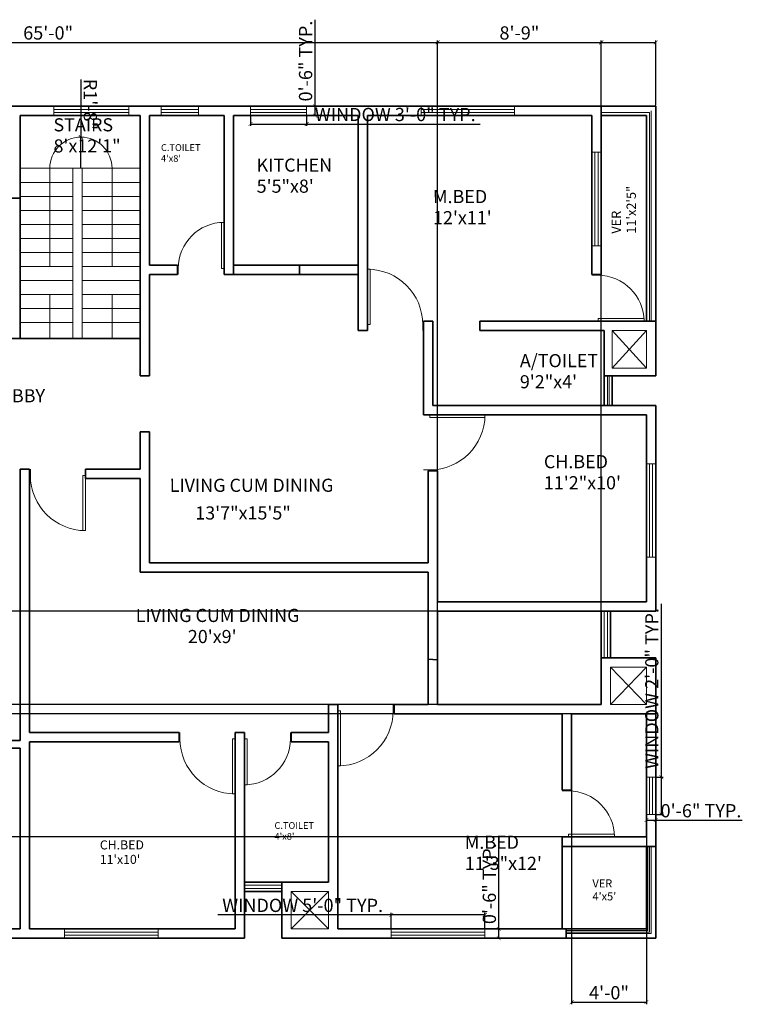
# Model space of a CAD drawing. Units: inches. Extents: x 3799 to 20199, y 1682 to 8087.
# Tile 3 of 30: x 6616 to 7080, y 1729 to 2361. Entities that reach past the tile are written whole.
import ezdxf

# ---------------------------------------------------------------- set-up
doc = ezdxf.new("R2010")
doc.units = ezdxf.units.IN
for name, color, linetype, lineweight in [('A-ANNO-DIMS', 2, 'Continuous', 18), ('A-AREA-IDEN', 7, 'Continuous', 18), ('A-DOOR', 3, 'Continuous', 18), ('A-FLOR-RAIL', 217, 'Continuous', 18), ('A-FLOR-SHFT', 8, 'Continuous', 18), ('A-FLOR-STRS', 41, 'Continuous', 18), ('A-GLAZ', 152, 'Continuous', 18), ('A-WALL', 7, 'Continuous', 35)]:
    doc.layers.add(name, color=color, linetype=linetype, lineweight=lineweight)
doc.styles.get("Standard").update_dxf_attribs({"font": 'arial.ttf'})
doc.dimstyles.new('ISO-25', dxfattribs={"dimtxt": 8.5, "dimasz": 2.5, "dimexe": 1.25, "dimexo": 0.625, "dimtad": 1, "dimdec": 0, "dimlunit": 3, "dimtxsty": 'Standard', "dimblk": 'ARCHTICK', "dimcen": 2.5, "dimadec": 0, "dimazin": 0, "dimtfac": 1, "dimtdec": 0, "dimtmove": 0, "dimatfit": 3, "dimfxl": 1, "dimarcsym": 0})

# ---------------------------------------------------------------- blocks, each defined once
blk = doc.blocks.new('*U16')
for p, q in [((0, 0), (0, -100)), ((900, 0), (900, -100))]:
    blk.add_line(p, q)
blk.add_lwpolyline([(0, 0), (0, 900), (43.75, 900), (43.75, 0)], close=True)
blk.add_arc((0, 0), 900, 0, 90)
blk = doc.blocks.new('*U17')
for p, q in [((-750, 0), (-750, -100)), ((0, 0), (0, -100))]:
    blk.add_line(p, q)
blk.add_lwpolyline([(0, 0), (0, 750), (-43.75, 750), (-43.75, 0)], close=True)
blk.add_arc((0, 0), 750, 90, 180)
blk = doc.blocks.new('*U11')
for p, q in [((-900, 0), (-900, 100)), ((0, 0), (0, 100))]:
    blk.add_line(p, q)
blk.add_lwpolyline([(0, 0), (0, -900), (-43.75, -900), (-43.75, 0)], close=True)
blk.add_arc((0, 0), 900, 180, 270)
blk = doc.blocks.new('*U13')
for p, q in [((0, 0), (0, 100)), ((750, 0), (750, 100))]:
    blk.add_line(p, q)
blk.add_lwpolyline([(0, 0), (0, -750), (43.75, -750), (43.75, 0)], close=True)
blk.add_arc((0, 0), 750, 270, 0)
blk = doc.blocks.new('*U14')
for p, q in [((0, 0), (0, 100)), ((900, 0), (900, 100))]:
    blk.add_line(p, q)
blk.add_lwpolyline([(0, 0), (0, -900), (43.75, -900), (43.75, 0)], close=True)
blk.add_arc((0, 0), 900, 270, 0)
blk = doc.blocks.new('*U15')
for p, q in [((0, 0), (0, 100)), ((750, 0), (750, 100))]:
    blk.add_line(p, q)
blk.add_lwpolyline([(0, 0), (0, -750), (43.75, -750), (43.75, 0)], close=True)
blk.add_arc((0, 0), 750, 270, 0)
blk = doc.blocks.new('*U18')
for p, q in [((-900, 0), (-900, 100)), ((0, 0), (0, 100))]:
    blk.add_line(p, q)
blk.add_lwpolyline([(0, 0), (0, -900), (-43.75, -900), (-43.75, 0)], close=True)
blk.add_arc((0, 0), 900, 180, 270)
blk = doc.blocks.new('*U19')
for p, q in [((0, 0), (0, 100)), ((750, 0), (750, 100))]:
    blk.add_line(p, q)
blk.add_lwpolyline([(0, 0), (0, -750), (43.75, -750), (43.75, 0)], close=True)
blk.add_arc((0, 0), 750, 270, 0)
blk = doc.blocks.new('WIN-60IN-6IN-FRAME')
for p, q in [((6, 60), (0, 60)), ((2, 60), (2, 0)), ((4, 60), (4, 0)), ((6, 0), (0, 0))]:
    blk.add_line(p, q)
blk = doc.blocks.new('WIN-24IN-6IN-FRAME')
for p, q in [((6, 24), (0, 24)), ((2, 24), (2, 0)), ((4, 24), (4, 0)), ((6, 0), (0, 0))]:
    blk.add_line(p, q)
blk = doc.blocks.new('WIN-48IN-6IN-FRAME')
for p, q in [((0, 0), (0, 6)), ((48, 4), (0, 4)), ((48, 2), (0, 2)), ((48, 0), (48, 6))]:
    blk.add_line(p, q)
blk = doc.blocks.new('WIN-36IN-6IN-FRAME')
for p, q in [((0, 0), (0, 6)), ((36, 4), (0, 4)), ((36, 2), (0, 2)), ((36, 0), (36, 6))]:
    blk.add_line(p, q)
blk = doc.blocks.new('SHAFT-24X24IN')
for p, q in [((0, 24), (0, 0)), ((24, 24), (0, 24)), ((0, 24), (24, 0)), ((0, 0), (24, 24)), ((24, 24), (24, 0)), ((0, 0), (24, 0))]:
    blk.add_line(p, q)
blk = doc.blocks.new('_ArchTick')
at = {"color": 0, "linetype": 'ByBlock', "const_width": 0.15}
blk.add_lwpolyline([(-0.5, -0.5), (0.5, 0.5)], dxfattribs=at)
blk = doc.blocks.new('*D268')
at = {"layer": 'A-ANNO-DIMS', "color": 0, "lineweight": -2, "transparency": 16777216}
for p, q in [((6854.93, 1786.05), (6743.62, 1786.05)), ((6854.93, 1777.67), (6854.93, 1787.3)), ((6914.93, 1786.05), (6854.93, 1786.05)), ((6914.93, 1777.67), (6914.93, 1787.3))]:
    blk.add_line(p, q, dxfattribs=at)
at = {"layer": 'Defpoints', "color": 0, "transparency": 16777216}
for p in [(6854.93, 1786.05), (6854.93, 1777.05), (6914.93, 1777.05)]:
    blk.add_point(p, dxfattribs=at)
at = {"layer": 'A-ANNO-DIMS', "color": 0, "lineweight": -2, "transparency": 16777216, "xscale": 2.5, "yscale": 2.5, "zscale": 2.5, "rotation": 180}
blk.add_blockref('_ArchTick', (6854.93, 1786.05), dxfattribs=at)
at = {"layer": 'A-ANNO-DIMS', "color": 0, "lineweight": -2, "transparency": 16777216, "xscale": 2.5, "yscale": 2.5, "zscale": 2.5}
blk.add_blockref('_ArchTick', (6914.93, 1786.05), dxfattribs=at)
at = {"layer": 'A-ANNO-DIMS', "color": 0, "transparency": 16777216, "insert": (6798.02, 1791.07), "char_height": 8.5, "attachment_point": 5}
blk.add_mtext('WINDOW 5\'-0" TYP.', dxfattribs=at)
blk = doc.blocks.new('*D269')
at = {"layer": 'A-ANNO-DIMS', "color": 0, "lineweight": -2, "transparency": 16777216}
for p, q in [((6923.93, 1777.05), (6923.93, 1832.61)), ((6915.55, 1777.05), (6925.18, 1777.05)), ((6923.93, 1771.05), (6923.93, 1777.05)), ((6915.55, 1771.05), (6925.18, 1771.05))]:
    blk.add_line(p, q, dxfattribs=at)
at = {"layer": 'Defpoints', "color": 0, "transparency": 16777216}
for p in [(6914.93, 1777.05), (6923.93, 1777.05), (6914.93, 1771.05)]:
    blk.add_point(p, dxfattribs=at)
at = {"layer": 'A-ANNO-DIMS', "color": 0, "lineweight": -2, "transparency": 16777216, "xscale": 2.5, "yscale": 2.5, "zscale": 2.5}
for p, rotation in [((6923.93, 1777.05), 90), ((6923.93, 1771.05), 270)]:
    blk.add_blockref('_ArchTick', p, dxfattribs=dict(at, rotation=rotation))
at = {"layer": 'A-ANNO-DIMS', "color": 0, "transparency": 16777216, "insert": (6918.96, 1806.08), "char_height": 8.5, "attachment_point": 5, "rotation": 90}
blk.add_mtext('0\'-6" TYP.', dxfattribs=at)
blk = doc.blocks.new('*D310')
at = {"layer": 'A-ANNO-DIMS', "color": 0, "lineweight": -2, "transparency": 16777216}
for p, q in [((7028.27, 1874.46), (7028.27, 1985.77)), ((7025.3, 1874.46), (7029.52, 1874.46)), ((7028.27, 1850.46), (7028.27, 1874.46)), ((7025.3, 1850.46), (7029.52, 1850.46))]:
    blk.add_line(p, q, dxfattribs=at)
at = {"layer": 'Defpoints', "color": 0, "transparency": 16777216}
for p in [(7024.67, 1874.46), (7028.27, 1874.46), (7024.67, 1850.46)]:
    blk.add_point(p, dxfattribs=at)
at = {"layer": 'A-ANNO-DIMS', "color": 0, "lineweight": -2, "transparency": 16777216, "xscale": 2.5, "yscale": 2.5, "zscale": 2.5}
for p, rotation in [((7028.27, 1874.46), 90), ((7028.27, 1850.46), 270)]:
    blk.add_blockref('_ArchTick', p, dxfattribs=dict(at, rotation=rotation))
at = {"layer": 'A-ANNO-DIMS', "color": 0, "transparency": 16777216, "insert": (7023.25, 1931.36), "char_height": 8.5, "attachment_point": 5, "rotation": 90}
blk.add_mtext('WINDOW 2\'-0" TYP.', dxfattribs=at)
blk = doc.blocks.new('*D311')
at = {"layer": 'A-ANNO-DIMS', "color": 0, "lineweight": -2, "transparency": 16777216}
for p, q in [((7018.67, 1849.83), (7018.67, 1845.61)), ((7018.67, 1846.86), (7024.67, 1846.86)), ((7024.67, 1849.83), (7024.67, 1845.61)), ((7024.67, 1846.86), (7080.24, 1846.86))]:
    blk.add_line(p, q, dxfattribs=at)
at = {"layer": 'Defpoints', "color": 0, "transparency": 16777216}
for p in [(7018.67, 1850.46), (7024.67, 1850.46), (7024.67, 1846.86)]:
    blk.add_point(p, dxfattribs=at)
at = {"layer": 'A-ANNO-DIMS', "color": 0, "lineweight": -2, "transparency": 16777216, "xscale": 2.5, "yscale": 2.5, "zscale": 2.5, "rotation": 180}
blk.add_blockref('_ArchTick', (7018.67, 1846.86), dxfattribs=at)
at = {"layer": 'A-ANNO-DIMS', "color": 0, "lineweight": -2, "transparency": 16777216, "xscale": 2.5, "yscale": 2.5, "zscale": 2.5}
blk.add_blockref('_ArchTick', (7024.67, 1846.86), dxfattribs=at)
at = {"layer": 'A-ANNO-DIMS', "color": 0, "transparency": 16777216, "insert": (7053.71, 1851.82), "char_height": 8.5, "attachment_point": 5}
blk.add_mtext('0\'-6" TYP.', dxfattribs=at)
blk = doc.blocks.new('*D336')
at = {"layer": 'A-ANNO-DIMS', "color": 0, "lineweight": -2, "transparency": 16777216}
for p, q in [((6764.57, 2298.42), (6764.57, 2292.4)), ((6800.57, 2298.42), (6800.57, 2292.4)), ((6764.57, 2293.65), (6800.57, 2293.65)), ((6800.57, 2293.65), (6911.88, 2293.65))]:
    blk.add_line(p, q, dxfattribs=at)
at = {"layer": 'Defpoints', "color": 0, "transparency": 16777216}
for p in [(6764.57, 2299.05), (6800.57, 2299.05), (6800.57, 2293.65)]:
    blk.add_point(p, dxfattribs=at)
at = {"layer": 'A-ANNO-DIMS', "color": 0, "lineweight": -2, "transparency": 16777216, "xscale": 2.5, "yscale": 2.5, "zscale": 2.5, "rotation": 180}
blk.add_blockref('_ArchTick', (6764.57, 2293.65), dxfattribs=at)
at = {"layer": 'A-ANNO-DIMS', "color": 0, "lineweight": -2, "transparency": 16777216, "xscale": 2.5, "yscale": 2.5, "zscale": 2.5}
blk.add_blockref('_ArchTick', (6800.57, 2293.65), dxfattribs=at)
at = {"layer": 'A-ANNO-DIMS', "color": 0, "transparency": 16777216, "insert": (6857.47, 2298.67), "char_height": 8.5, "attachment_point": 5}
blk.add_mtext('WINDOW 3\'-0" TYP.', dxfattribs=at)
blk = doc.blocks.new('*D337')
at = {"layer": 'A-ANNO-DIMS', "color": 0, "lineweight": -2, "transparency": 16777216}
for p, q in [((6805.97, 2305.05), (6805.97, 2360.61)), ((6801.19, 2305.05), (6807.22, 2305.05)), ((6805.97, 2299.05), (6805.97, 2305.05)), ((6801.19, 2299.05), (6807.22, 2299.05))]:
    blk.add_line(p, q, dxfattribs=at)
at = {"layer": 'Defpoints', "color": 0, "transparency": 16777216}
for p in [(6800.57, 2305.05), (6805.97, 2305.05), (6800.57, 2299.05)]:
    blk.add_point(p, dxfattribs=at)
at = {"layer": 'A-ANNO-DIMS', "color": 0, "lineweight": -2, "transparency": 16777216, "xscale": 2.5, "yscale": 2.5, "zscale": 2.5}
for p, rotation in [((6805.97, 2305.05), 90), ((6805.97, 2299.05), 270)]:
    blk.add_blockref('_ArchTick', p, dxfattribs=dict(at, rotation=rotation))
at = {"layer": 'A-ANNO-DIMS', "color": 0, "transparency": 16777216, "insert": (6801, 2334.08), "char_height": 8.5, "attachment_point": 5, "rotation": 90}
blk.add_mtext('0\'-6" TYP.', dxfattribs=at)
blk = doc.blocks.new('*D356')
at = {"layer": 'A-ANNO-DIMS', "color": 0, "lineweight": -2, "transparency": 16777216}
for p, q in [((6244.67, 2305.67), (6244.67, 2347.3)), ((6244.67, 2346.05), (7024.67, 2346.05)), ((7024.67, 2305.67), (7024.67, 2347.3))]:
    blk.add_line(p, q, dxfattribs=at)
at = {"layer": 'Defpoints', "color": 0, "transparency": 16777216}
for p in [(7024.67, 2346.05), (6244.67, 2305.05), (7024.67, 2305.05)]:
    blk.add_point(p, dxfattribs=at)
at = {"layer": 'A-ANNO-DIMS', "color": 0, "lineweight": -2, "transparency": 16777216, "xscale": 2.5, "yscale": 2.5, "zscale": 2.5, "rotation": 180}
blk.add_blockref('_ArchTick', (6244.67, 2346.05), dxfattribs=at)
at = {"layer": 'A-ANNO-DIMS', "color": 0, "lineweight": -2, "transparency": 16777216, "xscale": 2.5, "yscale": 2.5, "zscale": 2.5}
blk.add_blockref('_ArchTick', (7024.67, 2346.05), dxfattribs=at)
at = {"layer": 'A-ANNO-DIMS', "color": 0, "transparency": 16777216, "insert": (6634.67, 2351.01), "char_height": 8.5, "attachment_point": 5}
blk.add_mtext('65\'-0"', dxfattribs=at)
blk = doc.blocks.new('*D367')
at = {"layer": 'A-ANNO-DIMS', "color": 0, "lineweight": -2, "transparency": 16777216}
for p, q in [((6884.67, 1921.67), (6884.67, 2347.3)), ((6884.67, 2346.05), (6989.67, 2346.05)), ((6989.67, 1921.67), (6989.67, 2347.3))]:
    blk.add_line(p, q, dxfattribs=at)
at = {"layer": 'Defpoints', "color": 0, "transparency": 16777216}
for p in [(6989.67, 2346.05), (6884.67, 1921.05), (6989.67, 1921.05)]:
    blk.add_point(p, dxfattribs=at)
at = {"layer": 'A-ANNO-DIMS', "color": 0, "lineweight": -2, "transparency": 16777216, "xscale": 2.5, "yscale": 2.5, "zscale": 2.5, "rotation": 180}
blk.add_blockref('_ArchTick', (6884.67, 2346.05), dxfattribs=at)
at = {"layer": 'A-ANNO-DIMS', "color": 0, "lineweight": -2, "transparency": 16777216, "xscale": 2.5, "yscale": 2.5, "zscale": 2.5}
blk.add_blockref('_ArchTick', (6989.67, 2346.05), dxfattribs=at)
at = {"layer": 'A-ANNO-DIMS', "color": 0, "transparency": 16777216, "insert": (6937.17, 2351.01), "char_height": 8.5, "attachment_point": 5}
blk.add_mtext('8\'-9"', dxfattribs=at)
blk = doc.blocks.new('*D368')
at = {"layer": 'A-ANNO-DIMS', "color": 0, "lineweight": -2, "transparency": 16777216}
for p, q in [((6989.05, 1981.05), (6202.42, 1981.05)), ((6203.67, 1921.05), (6203.67, 1981.05)), ((6989.05, 1921.05), (6202.42, 1921.05))]:
    blk.add_line(p, q, dxfattribs=at)
at = {"layer": 'Defpoints', "color": 0, "transparency": 16777216}
for p in [(6203.67, 1981.05), (6989.67, 1981.05), (6989.67, 1921.05)]:
    blk.add_point(p, dxfattribs=at)
at = {"layer": 'A-ANNO-DIMS', "color": 0, "lineweight": -2, "transparency": 16777216, "xscale": 2.5, "yscale": 2.5, "zscale": 2.5}
for p, rotation in [((6203.67, 1981.05), 90), ((6203.67, 1921.05), 270)]:
    blk.add_blockref('_ArchTick', p, dxfattribs=dict(at, rotation=rotation))
at = {"layer": 'A-ANNO-DIMS', "color": 0, "transparency": 16777216, "insert": (6198.71, 1951.05), "char_height": 8.5, "attachment_point": 5, "rotation": 90}
blk.add_mtext('5\'-0"', dxfattribs=at)
blk = doc.blocks.new('*D369')
at = {"layer": 'A-ANNO-DIMS', "color": 0, "lineweight": -2, "transparency": 16777216}
for p, q in [((6970.67, 1914.42), (6970.67, 1728.8)), ((7018.67, 1914.42), (7018.67, 1728.8)), ((6970.67, 1730.05), (7018.67, 1730.05))]:
    blk.add_line(p, q, dxfattribs=at)
at = {"layer": 'Defpoints', "color": 0, "transparency": 16777216}
for p in [(6970.67, 1915.05), (7018.67, 1915.05), (7018.67, 1730.05)]:
    blk.add_point(p, dxfattribs=at)
at = {"layer": 'A-ANNO-DIMS', "color": 0, "lineweight": -2, "transparency": 16777216, "xscale": 2.5, "yscale": 2.5, "zscale": 2.5, "rotation": 180}
blk.add_blockref('_ArchTick', (6970.67, 1730.05), dxfattribs=at)
at = {"layer": 'A-ANNO-DIMS', "color": 0, "lineweight": -2, "transparency": 16777216, "xscale": 2.5, "yscale": 2.5, "zscale": 2.5}
blk.add_blockref('_ArchTick', (7018.67, 1730.05), dxfattribs=at)
at = {"layer": 'A-ANNO-DIMS', "color": 0, "transparency": 16777216, "insert": (6994.67, 1735.01), "char_height": 8.5, "attachment_point": 5}
blk.add_mtext('4\'-0"', dxfattribs=at)
blk = doc.blocks.new('*D370')
at = {"layer": 'A-ANNO-DIMS', "color": 0, "lineweight": -2, "transparency": 16777216}
for p, q in [((7018.05, 1915.05), (6202.42, 1915.05)), ((6203.67, 1836.05), (6203.67, 1915.05)), ((7018.05, 1836.05), (6202.42, 1836.05))]:
    blk.add_line(p, q, dxfattribs=at)
at = {"layer": 'Defpoints', "color": 0, "transparency": 16777216}
for p in [(6203.67, 1915.05), (7018.67, 1915.05), (7018.67, 1836.05)]:
    blk.add_point(p, dxfattribs=at)
at = {"layer": 'A-ANNO-DIMS', "color": 0, "lineweight": -2, "transparency": 16777216, "xscale": 2.5, "yscale": 2.5, "zscale": 2.5}
for p, rotation in [((6203.67, 1915.05), 90), ((6203.67, 1836.05), 270)]:
    blk.add_blockref('_ArchTick', p, dxfattribs=dict(at, rotation=rotation))
at = {"layer": 'A-ANNO-DIMS', "color": 0, "transparency": 16777216, "insert": (6198.71, 1875.55), "char_height": 8.5, "attachment_point": 5, "rotation": 90}
blk.add_mtext('6\'-7"', dxfattribs=at)
blk = doc.blocks.new('*D385')
at = {"layer": 'A-ANNO-DIMS', "color": 0, "lineweight": -2, "transparency": 16777216}
for p in [(6655.67, 2322.2), (6655.68, 2265.22)]:
    blk.add_line(p, (6655.68, 2285.22), dxfattribs=at)
at = {"layer": 'Defpoints', "color": 0, "transparency": 16777216}
for p in [(6655.68, 2285.22), (6655.68, 2265.22)]:
    blk.add_point(p, dxfattribs=at)
at = {"layer": 'A-ANNO-DIMS', "color": 0, "lineweight": -2, "transparency": 16777216, "xscale": 2.5, "yscale": 2.5, "zscale": 2.5, "rotation": 270.0003322570112}
blk.add_blockref('_ArchTick', (6655.68, 2285.22), dxfattribs=at)
at = {"layer": 'A-ANNO-DIMS', "color": 0, "transparency": 16777216, "insert": (6660.64, 2306.21), "char_height": 8.5, "attachment_point": 5, "rotation": 270.00033}
blk.add_mtext('R1\'-8"', dxfattribs=at)

msp = doc.modelspace()

# ---------------------------------------------------------------- linework, layer by layer
at = {"layer": 'A-FLOR-RAIL'}
for p, q in [((7020.67, 2301.05), (6989.67, 2301.05)), ((7020.67, 2167.05), (7020.67, 2301.05)), ((7021.67, 2167.05), (7021.67, 2302.05)), ((7019.67, 1776.05), (7019.67, 1830.05)), ((7020.67, 1775.05), (7020.67, 1830.05)), ((7021.67, 1774.05), (7021.67, 1830.05)), ((6967.17, 1776.05), (7019.67, 1776.05)), ((6967.17, 1775.05), (7020.67, 1775.05)), ((6967.17, 1775.05), (7018.67, 1775.05)), ((6967.17, 1774.05), (7021.67, 1774.05))]:
    msp.add_line(p, q, dxfattribs=at)
at = {"layer": 'A-FLOR-SHFT'}
for p, q in [((7018.67, 2161.05), (6996.67, 2161.05)), ((6996.67, 2161.05), (6996.67, 2137.05)), ((6996.67, 2161.05), (7018.67, 2137.05)), ((7018.67, 2161.05), (6996.67, 2137.05)), ((7018.67, 2161.05), (7018.67, 2137.05)), ((7018.67, 2137.05), (6996.67, 2137.05)), ((7018.67, 1945.05), (6995.67, 1945.05)), ((6995.67, 1945.05), (6995.67, 1921.05)), ((6995.67, 1945.05), (7018.67, 1921.05)), ((6995.67, 1921.05), (7018.67, 1945.05)), ((7018.67, 1921.05), (7018.67, 1945.05)), ((7018.67, 1921.05), (6995.67, 1921.05))]:
    msp.add_line(p, q, dxfattribs=at)
at = {"layer": 'A-FLOR-STRS'}
for p, q in [((6616.67, 2265.22), (6693.67, 2265.22)), ((6635.67, 2265.22), (6635.67, 2202.22)), ((6650.58, 2265.22), (6650.58, 2156.05)), ((6656.58, 2265.22), (6656.58, 2156.05)), ((6675.68, 2265.22), (6675.68, 2202.22)), ((6616.67, 2256.22), (6650.58, 2256.22)), ((6656.58, 2256.22), (6693.67, 2256.22)), ((6616.67, 2247.22), (6650.58, 2247.22)), ((6656.58, 2247.22), (6693.67, 2247.22)), ((6616.67, 2238.22), (6650.58, 2238.22)), ((6656.58, 2238.22), (6693.67, 2238.22)), ((6616.67, 2229.22), (6650.58, 2229.22)), ((6656.58, 2229.22), (6693.67, 2229.22)), ((6616.67, 2220.22), (6650.58, 2220.22)), ((6656.58, 2220.22), (6693.67, 2220.22)), ((6616.67, 2211.22), (6650.58, 2211.22)), ((6656.58, 2211.22), (6693.67, 2211.22)), ((6616.67, 2202.22), (6650.58, 2202.22)), ((6656.58, 2202.22), (6693.67, 2202.22)), ((6616.67, 2193.22), (6650.58, 2193.22)), ((6656.58, 2193.22), (6693.67, 2193.22)), ((6616.67, 2184.22), (6650.58, 2184.22)), ((6635.67, 2184.22), (6635.67, 2156.05)), ((6656.58, 2184.22), (6693.67, 2184.22)), ((6675.68, 2184.22), (6675.68, 2156.05)), ((6616.67, 2175.22), (6650.58, 2175.22)), ((6656.58, 2175.22), (6693.67, 2175.22)), ((6616.67, 2166.22), (6650.58, 2166.22)), ((6656.58, 2166.22), (6693.67, 2166.22))]:
    msp.add_line(p, q, dxfattribs=at)
msp.add_arc((6655.68, 2265.22), 20, 360, 180, dxfattribs=at)
at = {"layer": 'A-GLAZ'}
for p, q in [((6993.67, 2132.05), (6993.67, 2113.05)), ((6994.67, 2132.05), (6994.67, 2113.05)), ((6991.67, 1981.05), (6991.67, 1951.05)), ((6993.67, 1981.05), (6993.67, 1951.05)), ((6760.67, 1805.05), (6784.67, 1805.05)), ((6760.67, 1803.05), (6784.67, 1803.05))]:
    msp.add_line(p, q, dxfattribs=at)
at = {"layer": 'A-WALL'}
for p, q in [((7024.67, 2305.05), (6244.67, 2305.05)), ((6989.67, 2197.05), (6989.67, 2305.05)), ((7024.67, 2132.05), (7024.67, 2305.05)), ((6693.67, 2299.05), (6616.67, 2299.05)), ((6616.67, 2246.05), (6616.67, 2299.05)), ((6693.67, 2299.05), (6693.67, 2132.05)), ((6699.67, 2299.05), (6699.67, 2203.05)), ((6747.67, 2299.05), (6699.67, 2299.05)), ((6747.67, 2299.05), (6747.67, 2197.05)), ((6753.67, 2299.05), (6753.67, 2197.05)), ((6833.67, 2299.05), (6753.67, 2299.05)), ((6833.67, 2161.05), (6833.67, 2299.05)), ((6839.67, 2161.05), (6839.67, 2299.05)), ((6983.67, 2299.05), (6839.67, 2299.05)), ((6983.67, 2197.05), (6983.67, 2299.05)), ((7018.67, 2299.05), (6989.67, 2299.05)), ((7018.67, 2167.05), (7018.67, 2299.05)), ((6616.67, 2246.05), (6538.67, 2246.05)), ((6616.67, 2246.05), (6616.67, 2156.05)), ((6717.67, 2203.05), (6699.67, 2203.05)), ((6717.67, 2203.05), (6717.67, 2197.05)), ((6833.67, 2203.05), (6753.67, 2203.05)), ((6795.97, 2203.05), (6795.97, 2197.05)), ((6717.67, 2197.05), (6699.67, 2197.05)), ((6699.67, 2197.05), (6699.67, 2132.05)), ((6833.67, 2197.05), (6747.67, 2197.05)), ((6989.67, 2197.05), (6983.67, 2197.05)), ((6875.67, 2161.05), (6875.67, 2167.05)), ((6881.67, 2167.05), (6875.67, 2167.05)), ((6881.67, 2161.05), (6881.67, 2167.05)), ((7024.67, 2167.05), (6911.67, 2167.05)), ((6911.67, 2161.05), (6911.67, 2167.05)), ((6536.67, 2156.05), (6693.67, 2156.05)), ((6839.67, 2161.05), (6833.67, 2161.05)), ((6875.67, 2161.05), (6875.67, 2107.05)), ((6881.67, 2161.05), (6881.67, 2113.05)), ((6991.67, 2161.05), (6911.67, 2161.05)), ((6991.67, 2161.05), (6991.67, 2113.05)), ((6693.67, 2132.05), (6699.67, 2132.05)), ((7018.67, 2132.05), (6991.67, 2132.05)), ((6996.67, 2132.05), (6996.67, 2113.05)), ((7018.67, 2132.05), (7024.67, 2132.05)), ((6989.67, 2113.05), (6881.67, 2113.05)), ((6983.67, 2113.05), (7018.67, 2113.05)), ((7018.67, 2113.05), (7024.67, 2113.05)), ((7024.67, 1981.05), (7024.67, 2113.05)), ((7018.67, 2107.05), (6875.67, 2107.05)), ((7018.67, 1987.05), (7018.67, 2107.05)), ((6693.67, 2096.05), (6699.67, 2096.05)), ((6693.67, 2096.05), (6693.67, 2072.05)), ((6699.67, 2096.05), (6699.67, 2012.05)), ((6616.67, 2072.05), (6616.67, 1898.05)), ((6616.67, 2072.05), (6622.67, 2072.05)), ((6622.67, 2072.05), (6622.67, 1903.05)), ((6658.67, 2072.05), (6658.67, 2066.05)), ((6658.67, 2072.05), (6693.67, 2072.05)), ((6884.67, 2071.05), (6878.67, 2071.05)), ((6878.67, 2012.05), (6878.67, 2071.05)), ((6884.67, 1987.05), (6884.67, 2071.05)), ((6658.67, 2066.05), (6693.67, 2066.05)), ((6693.67, 2066.05), (6693.67, 2006.05)), ((6878.67, 2012.05), (6699.67, 2012.05)), ((6878.67, 2006.05), (6693.67, 2006.05)), ((6878.67, 1921.05), (6878.67, 2006.05)), ((7018.67, 1987.05), (6884.67, 1987.05)), ((6884.67, 1921.05), (6884.67, 1981.05)), ((7024.67, 1981.05), (6884.67, 1981.05)), ((6989.67, 1981.05), (6989.67, 1921.05)), ((6995.67, 1981.05), (6995.67, 1951.05)), ((6884.67, 1949.85), (6878.67, 1950.2)), ((7024.67, 1951.05), (6989.67, 1951.05)), ((7024.67, 1771.05), (7024.67, 1951.05)), ((6814.67, 1921.05), (6820.67, 1921.05)), ((6814.67, 1903.05), (6814.67, 1921.05)), ((6820.67, 1777.05), (6820.67, 1921.05)), ((6856.67, 1915.05), (6856.67, 1921.05)), ((6856.67, 1921.05), (6878.67, 1921.05)), ((6878.67, 1915.05), (6856.67, 1915.05)), ((6964.67, 1915.05), (6878.67, 1915.05)), ((6989.67, 1921.05), (6884.67, 1921.05)), ((6964.67, 1866.05), (6964.67, 1915.05)), ((7024.67, 1915.05), (6970.67, 1915.05)), ((6970.67, 1866.05), (6970.67, 1915.05)), ((7018.67, 1836.05), (7018.67, 1915.05)), ((6622.67, 1903.05), (6718.67, 1903.05)), ((6718.67, 1903.05), (6718.67, 1897.05)), ((6754.67, 1903.05), (6754.67, 1777.05)), ((6754.67, 1903.05), (6760.67, 1903.05)), ((6760.67, 1903.05), (6760.67, 1807.05)), ((6790.67, 1903.05), (6790.67, 1897.05)), ((6790.67, 1903.05), (6814.67, 1903.05)), ((6616.67, 1898.05), (6532.67, 1898.05)), ((6622.67, 1897.05), (6718.67, 1897.05)), ((6622.67, 1897.05), (6622.67, 1777.05)), ((6790.67, 1897.05), (6814.67, 1897.05)), ((6814.67, 1807.05), (6814.67, 1897.05)), ((6616.67, 1893.05), (6532.67, 1893.05)), ((6616.67, 1893.05), (6616.67, 1777.05)), ((6970.67, 1866.05), (6964.67, 1866.05)), ((7018.67, 1836.05), (6964.67, 1836.05)), ((6964.67, 1830.05), (6964.67, 1836.05)), ((7024.67, 1830.05), (6964.67, 1830.05)), ((6964.67, 1830.05), (6964.67, 1777.05)), ((7018.67, 1777.05), (7018.67, 1830.05)), ((6760.67, 1807.05), (6814.67, 1807.05)), ((6760.67, 1807.05), (6760.67, 1771.05)), ((6760.67, 1801.05), (6784.67, 1801.05)), ((6784.67, 1771.05), (6784.67, 1807.05)), ((6496.67, 1777.05), (6616.67, 1777.05)), ((6622.67, 1777.05), (6754.67, 1777.05)), ((6820.67, 1777.05), (7018.67, 1777.05)), ((6967.17, 1777.05), (6967.17, 1771.05)), ((6491.67, 1771.05), (6760.67, 1771.05)), ((6784.67, 1771.05), (7024.67, 1771.05))]:
    msp.add_line(p, q, dxfattribs=at)

# ---------------------------------------------------------------- block references
at = {"layer": 'A-DOOR', "xscale": 0.0393700787401575, "yscale": 0.0393700787401575, "zscale": 0.0393700787401575}
for name, p in [('*U17', (6747.67, 2200.99)), ('*U16', (6839.67, 2164.99)), ('*U11', (6658.67, 2068.11)), ('*U14', (6820.67, 1917.11)), ('*U11', (6754.67, 1899.11)), ('*U13', (6760.67, 1899.11))]:
    msp.add_blockref(name, p, dxfattribs=at)
at = {"layer": 'A-DOOR', "xscale": 0.0393700787401575, "yscale": 0.0393700787401575, "zscale": 0.0393700787401575, "rotation": 90}
for name, p in [('*U19', (6987.61, 2167.05)), ('*U18', (6879.61, 2107.05)), ('*U15', (6968.61, 1836.05))]:
    msp.add_blockref(name, p, dxfattribs=at)
at = {"layer": 'A-FLOR-SHFT'}
msp.add_blockref('SHAFT-24X24IN', (6790.68, 1777.05), dxfattribs=at)
at = {"layer": 'A-GLAZ'}
for name, p in [('WIN-48IN-6IN-FRAME', (6638.39, 2299.05)), ('WIN-36IN-6IN-FRAME', (6764.57, 2299.05)), ('WIN-60IN-6IN-FRAME', (6983.67, 2215.51)), ('WIN-60IN-6IN-FRAME', (7018.67, 2015.61)), ('WIN-24IN-6IN-FRAME', (7018.67, 1850.45))]:
    msp.add_blockref(name, p, dxfattribs=at)
at = {"layer": 'A-GLAZ', "rotation": 90}
for name, p in [('WIN-24IN-6IN-FRAME', (6731.14, 2299.05)), ('WIN-60IN-6IN-FRAME', (6934.01, 2299.05)), ('WIN-60IN-6IN-FRAME', (6705.26, 1771.05)), ('WIN-60IN-6IN-FRAME', (6914.93, 1771.05))]:
    msp.add_blockref(name, p, dxfattribs=at)

# ---------------------------------------------------------------- texts
at = {"layer": 'A-AREA-IDEN'}
for s, height, rotation, p in [('STAIRS', 8.428, 0.03333, (6638.09, 2288.92)), ('8\'x12\'1"', 8.428, 0.03333, (6638.1, 2275.38)), ('C.TOILET', 4.344, 0.03333, (6707.09, 2276.37)), ("4'x8'", 4.344, 0.03333, (6707.09, 2269.39)), ('KITCHEN', 8.428, 0.03333, (6768.48, 2263.07)), ('5\'5"x8\'', 8.428, 0.03333, (6768.49, 2249.53)), ('M.BED', 8.428, 0.03333, (6881.71, 2242.87)), ('11\'x2\'5"', 5.992, 90.03333, (7011.94, 2223.29)), ("12'x11'", 8.428, 0.03333, (6881.72, 2229.33)), ('VER', 5.992, 90.03333, (7002.31, 2223.28)), ('A/TOILET', 8.428, 0.03333, (6937.45, 2137.56)), ('9\'2"x4\'', 8.428, 0.03333, (6937.46, 2124.02)), ('LOBBY', 8.428, 0.03333, (6596.66, 2115.03)), ('CH.BED', 8.428, 0.03333, (6952.87, 2072.72)), ('11\'2"x10\'', 8.428, 0.03333, (6952.88, 2059.18)), ('LIVING CUM DINING', 8.4277, 0.03333, (6712.68, 2057.54)), ('13\'7"x15\'5"', 8.4277, 0.03333, (6729.12, 2039.81)), ('LIVING CUM DINING', 8.4277, 0.03333, (6690.86, 1974)), ("             20'x9'", 8.4277, 0.03333, (6690.87, 1960.47)), ('C.TOILET', 4.344, 0.03333, (6779.94, 1841.24)), ('CH.BED', 5.798, 0.03333, (6667.85, 1828.08)), ("4'x8'", 4.344, 0.03333, (6779.95, 1834.26)), ('M.BED', 8.428, 0.03333, (6902.12, 1828.45)), ("11'x10'", 5.798, 0.03333, (6667.86, 1818.77)), ('11\'3"x12\'', 8.428, 0.03333, (6902.13, 1814.92)), ('VER', 5.177, 0.03333, (6984.04, 1803.67)), ("4'x5'", 5.177, 0.03333, (6984.04, 1795.35))]:
    msp.add_text(s, height=height, rotation=rotation, dxfattribs=at).set_placement(p)

# ---------------------------------------------------------------- dimensions: what is measured, and where the dimension line sits
at = {"layer": 'A-ANNO-DIMS'}
for base, p1, p2, angle, text, picture, middle in [((6805.97, 2305.05), (6800.57, 2299.05), (6800.57, 2305.05), 90, '<> TYP.', '*D337', (6801, 2334.08)), ((7028.27, 1874.46), (7024.67, 1850.46), (7024.67, 1874.46), 90, 'WINDOW <> TYP.', '*D310', (7023.25, 1931.36)), ((6923.93, 1777.05), (6914.93, 1771.05), (6914.93, 1777.05), 90, '<> TYP.', '*D269', (6918.96, 1806.08)), ((6854.93, 1786.05), (6914.93, 1777.05), (6854.93, 1777.05), 180, 'WINDOW <> TYP.', '*D268', (6798.02, 1791.07))]:
    dim = msp.add_linear_dim(base=base, p1=p1, p2=p2, angle=angle, text=text, dimstyle='ISO-25', override={"dimdec": 1, "dimlfac": 1, "dimrnd": 0, "dimzin": 1, "dimdsep": 46, "dimlunit": 4, "dimfrac": 2}, dxfattribs=at)
    dim.commit()
    dim.dimension.update_dxf_attribs({"geometry": picture, "text_midpoint": middle})
for base, p1, p2, picture, middle in [((7024.67, 2346.05), (6244.67, 2305.05), (7024.67, 2305.05), '*D356', (6634.67, 2351.01)), ((6989.67, 2346.05), (6884.67, 1921.05), (6989.67, 1921.05), '*D367', (6937.17, 2351.01)), ((7018.67, 1730.05), (6970.67, 1915.05), (7018.67, 1915.05), '*D369', (6994.67, 1735.01))]:
    dim = msp.add_linear_dim(base=base, p1=p1, p2=p2, dimstyle='ISO-25', override={"dimdec": 1, "dimlfac": 1, "dimrnd": 0, "dimzin": 1, "dimdsep": 46, "dimlunit": 4, "dimfrac": 2}, dxfattribs=at)
    dim.commit()
    dim.dimension.update_dxf_attribs({"geometry": picture, "text_midpoint": middle})
dim = msp.add_radius_dim(center=(6655.68, 2265.22), mpoint=(6655.68, 2285.22), dimstyle='ISO-25', override={"dimdec": 1, "dimlfac": 1, "dimrnd": 0, "dimzin": 1, "dimdsep": 46, "dimlunit": 4, "dimfrac": 2}, dxfattribs=at)
dim.commit()
dim.dimension.update_dxf_attribs({"geometry": '*D385', "text_midpoint": (6660.64, 2306.21)})
for base, p1, p2, text, picture, middle in [((6800.57, 2293.65), (6764.57, 2299.05), (6800.57, 2299.05), 'WINDOW <> TYP.', '*D336', (6857.47, 2298.67)), ((7024.67, 1846.86), (7018.67, 1850.46), (7024.67, 1850.46), '<> TYP.', '*D311', (7053.71, 1851.82))]:
    dim = msp.add_linear_dim(base=base, p1=p1, p2=p2, text=text, dimstyle='ISO-25', override={"dimdec": 1, "dimlfac": 1, "dimrnd": 0, "dimzin": 1, "dimdsep": 46, "dimlunit": 4, "dimfrac": 2}, dxfattribs=at)
    dim.commit()
    dim.dimension.update_dxf_attribs({"geometry": picture, "text_midpoint": middle})
for base, p1, p2, picture, middle in [((6203.67, 1981.05), (6989.67, 1921.05), (6989.67, 1981.05), '*D368', (6198.71, 1951.05)), ((6203.67, 1915.05), (7018.67, 1836.05), (7018.67, 1915.05), '*D370', (6198.71, 1875.55))]:
    dim = msp.add_linear_dim(base=base, p1=p1, p2=p2, angle=90, dimstyle='ISO-25', override={"dimdec": 1, "dimlfac": 1, "dimrnd": 0, "dimzin": 1, "dimdsep": 46, "dimlunit": 4, "dimfrac": 2}, dxfattribs=at)
    dim.commit()
    dim.dimension.update_dxf_attribs({"geometry": picture, "text_midpoint": middle})

doc.saveas('drawing.dxf')
